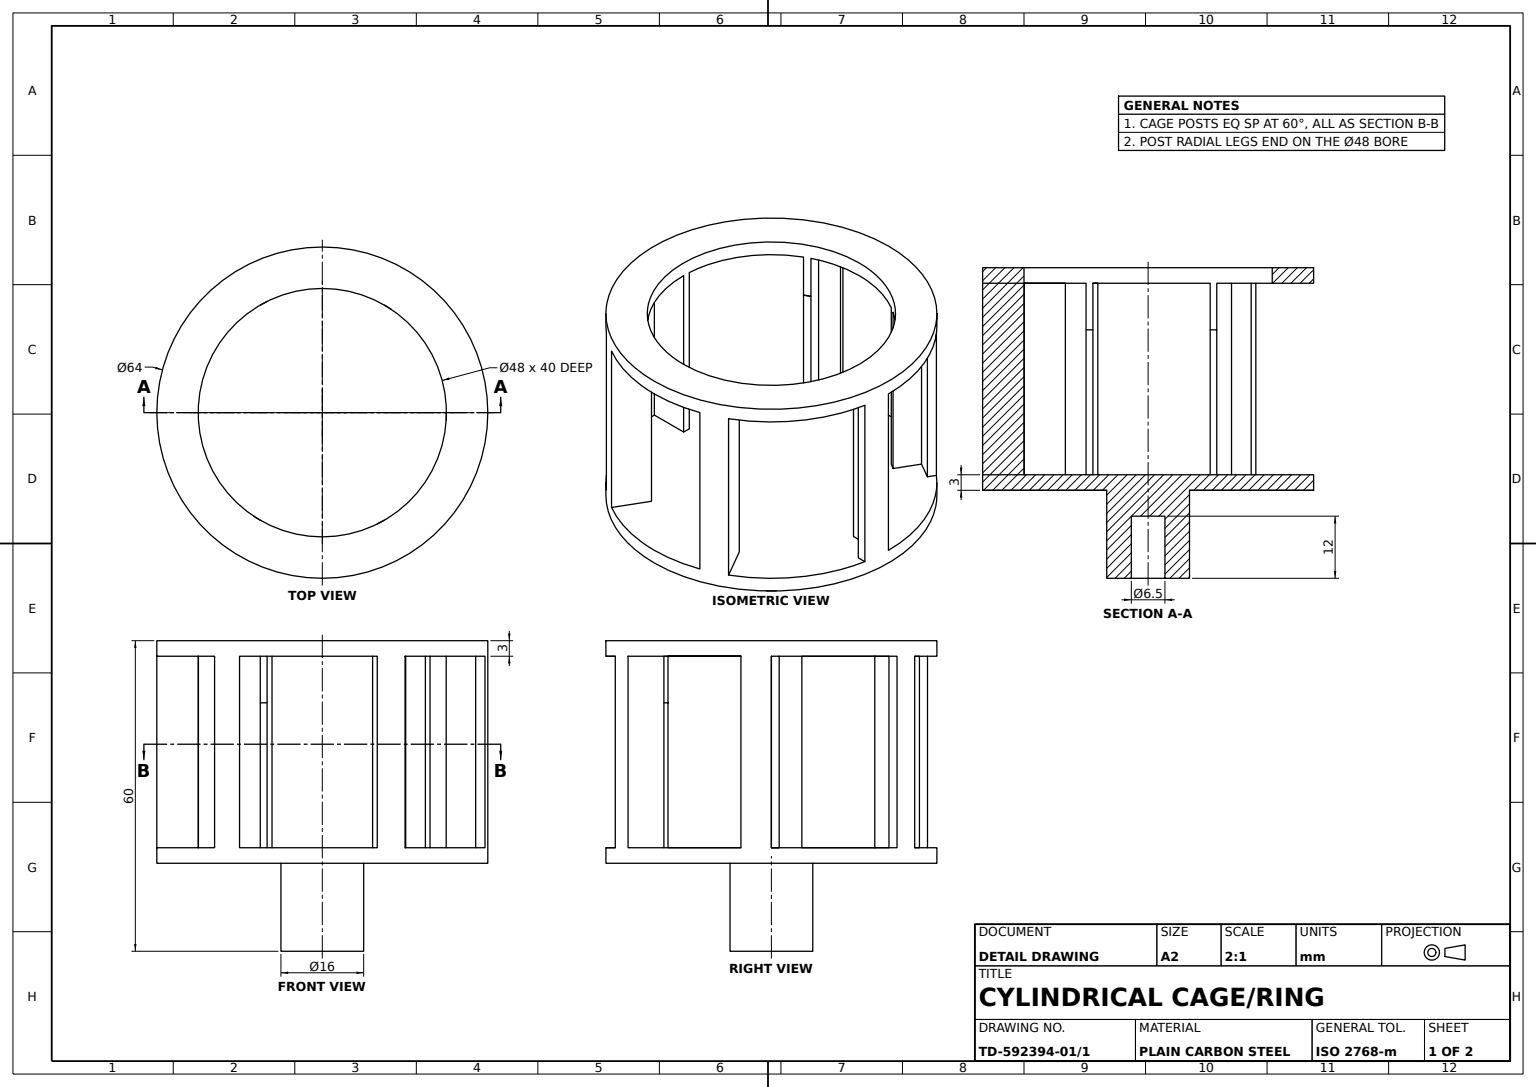
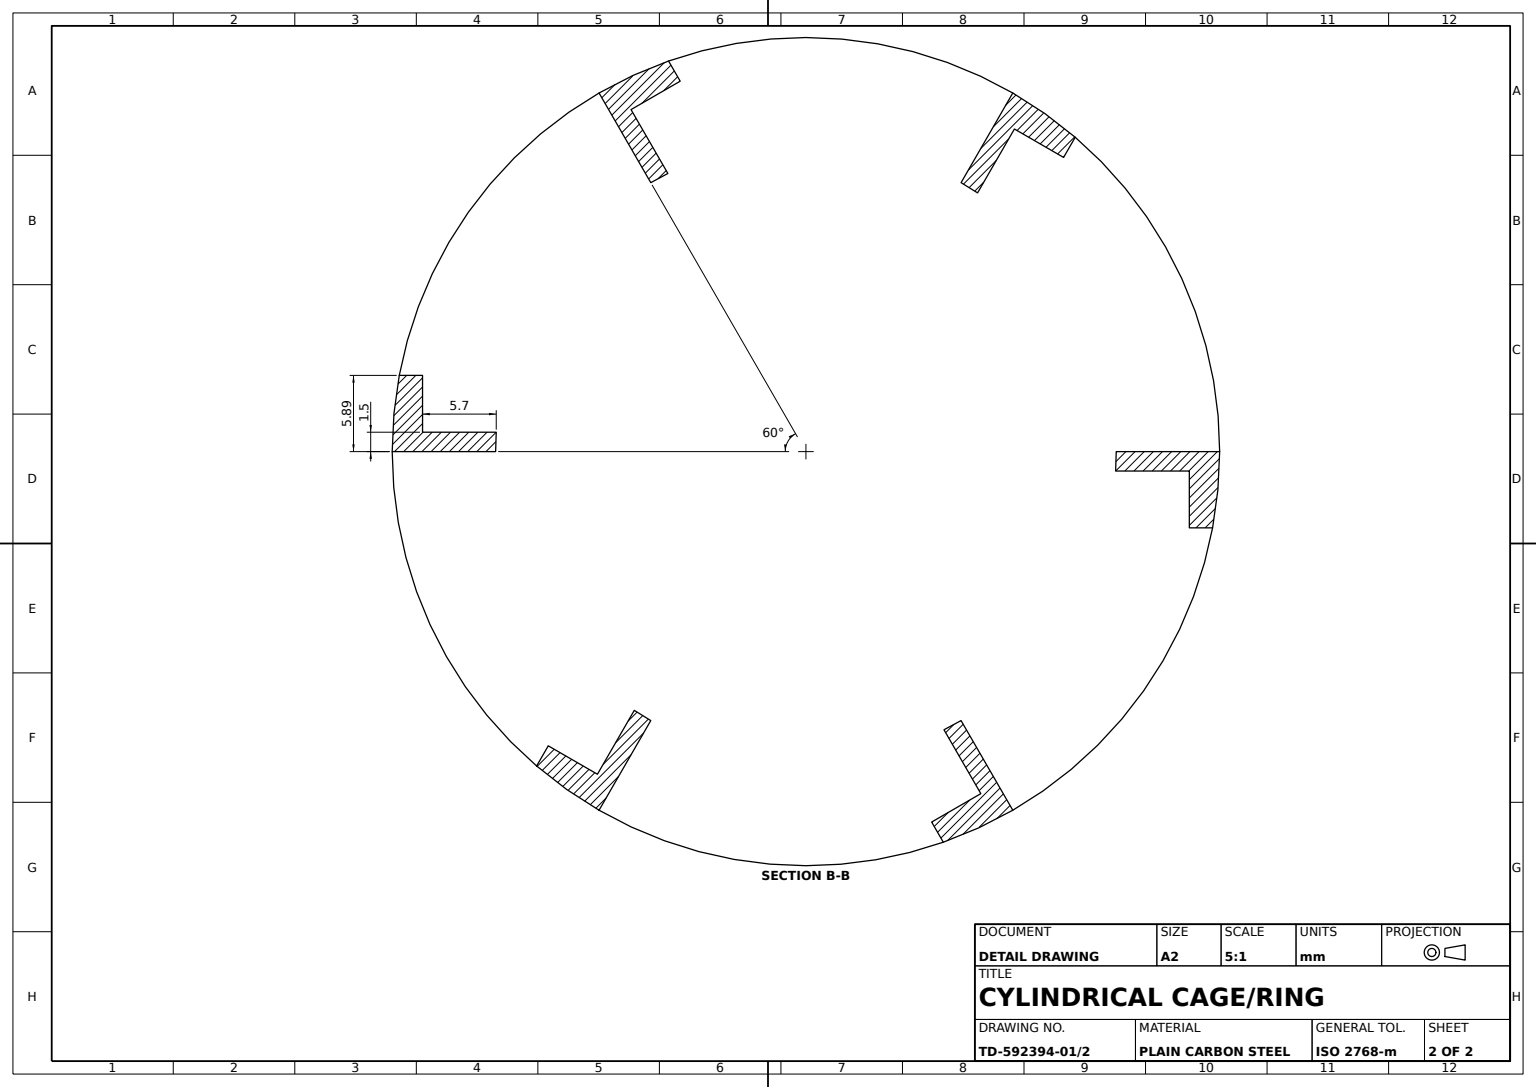
SolidWorks part; units mm, degrees
material "Plain Carbon Steel"
ref_plane "Front Plane" through (0, 0, 0) normal (0, 0, 1) x (1, 0, 0)
ref_plane "Top Plane" through (0, 0, 0) normal (0, 1, 0) x (1, 0, 0)
ref_plane "Right Plane" through (0, 0, 0) normal (1, 0, 0) x (0, 0, -1)
sketch "Base Disc Sketch" plane through (0, 0, 0) normal (0, 1, 0) x (1, 0, 0)
  circle A0 centre (0, 0) radius 32
  dimension "D1" = 64
extrude "Base Disc Ø64" add sketch "Base Disc Sketch" along normal blind 3
sketch "Cage Posts Sketch" plane through (0, 3, 0) normal (0, 1, 0) x (1, 0, 0)
  line L0 (-24, 0) -> (-32, 0)
  line L1 (-31.4531, 5.891) -> (-29.6531, 5.891)
  line L2 (-29.6531, 5.891) -> (-29.6531, 1.5)
  line L3 (-29.6531, 1.5) -> (-23.9531, 1.5)
  line L4 (-23.9531, 1.5) -> (-24, 0)
  line L5 (-10.6775, 21.494) -> (-12, 20.7846)
  line L6 (-12, 20.7846) -> (-16, 27.7128)
  line L7 (-10.6248, 30.1847) -> (-9.7248, 28.6258)
  line L8 (-9.7248, 28.6258) -> (-13.5275, 26.4303)
  line L9 (-13.5275, 26.4303) -> (-10.6775, 21.494)
  line L10 (13.2756, 19.994) -> (12, 20.7846)
  line L11 (12, 20.7846) -> (16, 27.7128)
  line L12 (20.8283, 24.2937) -> (19.9283, 22.7348)
  line L13 (19.9283, 22.7348) -> (16.1256, 24.9303)
  line L14 (16.1256, 24.9303) -> (13.2756, 19.994)
  line L15 (23.9531, -1.5) -> (24, 0)
  line L16 (24, 0) -> (32, 0)
  line L17 (31.4531, -5.891) -> (29.6531, -5.891)
  line L18 (29.6531, -5.891) -> (29.6531, -1.5)
  line L19 (29.6531, -1.5) -> (23.9531, -1.5)
  line L20 (10.6775, -21.494) -> (12, -20.7846)
  line L21 (12, -20.7846) -> (16, -27.7128)
  line L22 (10.6248, -30.1847) -> (9.7248, -28.6258)
  line L23 (9.7248, -28.6258) -> (13.5275, -26.4303)
  line L24 (13.5275, -26.4303) -> (10.6775, -21.494)
  line L25 (-13.2756, -19.994) -> (-12, -20.7846)
  line L26 (-12, -20.7846) -> (-16, -27.7128)
  line L27 (-20.8283, -24.2937) -> (-19.9283, -22.7348)
  line L28 (-19.9283, -22.7348) -> (-16.1256, -24.9303)
  line L29 (-16.1256, -24.9303) -> (-13.2756, -19.994)
  arc A0 (-23.9531, 1.5) -> (-24, 0) centre (0, 0) ccw
  circle A1 centre (0, 0) radius 32 construction
  arc A2 (-32, 0) -> (-31.4531, 5.891) centre (0, 0) cw
  arc A3 (-16, 27.7128) -> (-10.6248, 30.1847) centre (0, 0) cw
  arc A4 (16, 27.7128) -> (20.8283, 24.2937) centre (0, 0) cw
  arc A5 (32, 0) -> (31.4531, -5.891) centre (0, 0) cw
  arc A6 (16, -27.7128) -> (10.6248, -30.1847) centre (0, 0) cw
  arc A7 (-16, -27.7128) -> (-20.8283, -24.2937) centre (0, 0) cw
  point P44 (0, 0)
  circle M13 centre (0, 0) radius 32
  dimension "D1" = 48
  dimension "D2" = 1.5
  dimension "D3" = 1.8
  dimension "D4" = 5.7
  dimension "D5" = 6
extrude "Cage Posts 6x" add sketch "Cage Posts Sketch" along normal blind 40 contours L29 L28 L27 L26 L25 M13 | L19 L18 L17 L16 L15 M13 | L14 L13 L12 L11 L10 M13 | A0 L3 L2 L1 L0 M13 | L23 L24 L20 L21 A6 L22 | A3 L7 L8 L9 L5 L6
sketch "Top Ring Sketch" plane through (0, 43, 0) normal (0, 1, 0) x (1, 0, 0)
  circle A0 centre (0, 0) radius 32
extrude "Top Ring" add sketch "Top Ring Sketch" against normal blind 3
sketch "Hub Sketch" plane through (0, 0, 0) normal (0, -1, 0) x (1, 0, 0)
  circle A0 centre (0, 0) radius 8
  dimension "D1" = 16
extrude "Hub Ø16" add sketch "Hub Sketch" along normal blind 17
sketch "Hub Bore Sketch" plane through (0, -17, 0) normal (0, -1, 0) x (1, 0, 0)
  circle A0 centre (0, 0) radius 3.25
  dimension "D1" = 6.5
extrude "Hub Bore Ø6.5" cut sketch "Hub Bore Sketch" against normal blind 12
sketch "Inner Recess Sketch" plane through (0, 43, 0) normal (0, 1, 0) x (1, 0, 0)
  circle A0 centre (0, 0) radius 24
  dimension "D1" = 48
extrude "Inner Recess Ø48" cut sketch "Inner Recess Sketch" against normal blind 12
